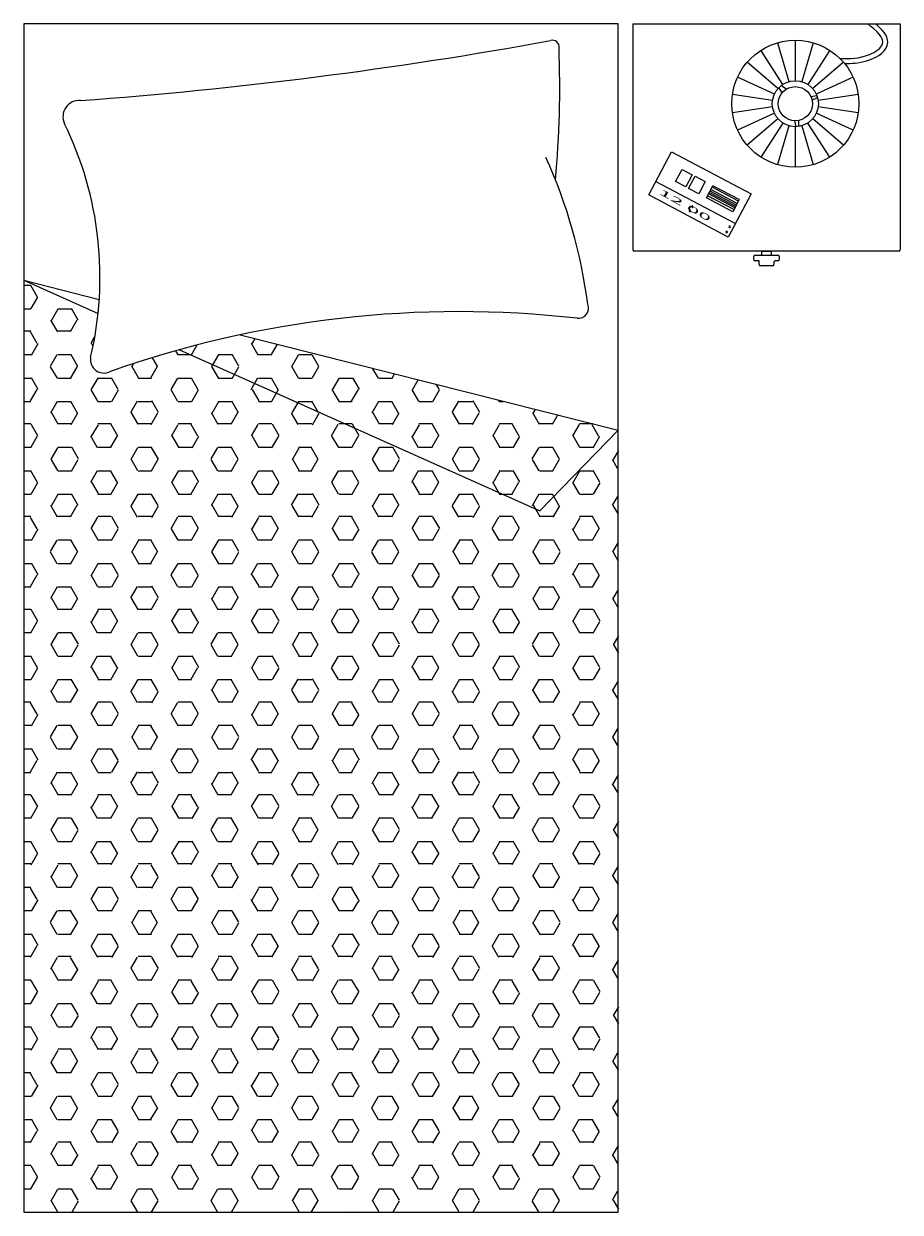
# Model space of a CAD drawing. Units: inches. Extents: x 1994 to 3075, y 3517 to 3950.
# Tile 12 of 58: x 1994.32638 to 1994.38593, y 3553.35463 to 3553.4354. Entities that reach past the tile are written whole.
import ezdxf

# ---------------------------------------------------------------- set-up
doc = ezdxf.new("R2010")
doc.units = ezdxf.units.IN
for name, color, linetype, lineweight in [('A-FURN-REFR', 8, 'Continuous', 13), ('A-FURN-REFR-PATT', 8, 'Continuous', 13), ('A-FURN-REFR-TEXT', 7, 'Continuous', 13)]:
    doc.layers.add(name, color=color, linetype=linetype, lineweight=lineweight)
doc.styles.get("Standard").update_dxf_attribs({"font": 'arial.ttf'})

msp = doc.modelspace()

# ---------------------------------------------------------------- hatches: boundary and pattern name
at = {"layer": 'A-FURN-REFR-PATT'}
h = msp.add_hatch(dxfattribs=at)
h.set_pattern_fill('HEX', color=256, scale=0.000286327845383, style=0)
h.set_pattern_definition([(180, (1995.655047321189, 3553.090100364233), (0, 0.0015745912670007), [0.0009090909090909, -0.0018181818181818]), (60, (1995.655047321189, 3553.090100364233), (0.0013636360377997, -0.0007872956335004), [0.0009090909090909, -0.0018181818181818]), (120, (1995.65413823028, 3553.090100364233), (0.0013636360377997, 0.0007872956335004), [0.0009090909090909, -0.0018181818181818])])
h.paths.add_polyline_path([(1994.326376891248, 3553.417965362907), (1994.331426744007, 3553.415710482533, -0.0305209839665435), (1994.33094919599, 3553.412850547023, 0.6531656006292759), (1994.332203126072, 3553.411747859217, -0.0174826565832849), (1994.336948128047, 3553.413245052134), (1994.361441213475, 3553.402308302044), (1994.366761804984, 3553.40777293816), (1994.366761804984, 3553.354629115022), (1994.326376891248, 3553.354629115022)])
h.paths.add_polyline_path([(1994.336948128047, 3553.413245052134, -0.0149090101017863), (1994.341069117673, 3553.414257309618), (1994.366761804984, 3553.40777293816), (1994.361441213475, 3553.402308302044)], flags=17)

# ---------------------------------------------------------------- linework, layer by layer
at = {"layer": 'A-FURN-REFR'}
for p, q in [((1994.326376891248, 3553.435398942494), (1994.326376891248, 3553.354629115022)), ((1994.366761804984, 3553.435398942494), (1994.326376891248, 3553.435398942494)), ((1994.366761804984, 3553.435398942494), (1994.326376891248, 3553.435398942494)), ((1994.326376891248, 3553.435398942494), (1994.326376891248, 3553.354629115022)), ((1994.366761804984, 3553.419954310977), (1994.366761804984, 3553.435398942494)), ((1994.367755092342, 3553.435398942494), (1994.385928303524, 3553.435398942494)), ((1994.367755092342, 3553.435398942494), (1994.385928303524, 3553.435398942494)), ((1994.367755092342, 3553.435398942494), (1994.367755092342, 3553.420048816135)), ((1994.385928303524, 3553.435398942494), (1994.385928303524, 3553.420048816135)), ((1994.37758513782, 3553.434108248894), (1994.3783607243, 3553.431466843914)), ((1994.378801208797, 3553.434283093505), (1994.378801208797, 3553.431530176024)), ((1994.378801208797, 3553.434283093505), (1994.378801208797, 3553.431530176024)), ((1994.380017279775, 3553.434108248894), (1994.379241693294, 3553.431466843914)), ((1994.377955925238, 3553.431281978377), (1994.376467585681, 3553.433597879934)), ((1994.381134831914, 3553.433597879934), (1994.379646492356, 3553.431281978377)), ((1994.377619606023, 3553.430990556118), (1994.375539089808, 3553.43279333368)), ((1994.382063327786, 3553.43279333368), (1994.379982811572, 3553.430990556118)), ((1994.377379013236, 3553.430616186435), (1994.374874871415, 3553.431759789686)), ((1994.382727546179, 3553.431759789686), (1994.380223404358, 3553.430616186435)), ((1994.377906583764, 3553.430702690964), (1994.377682333013, 3553.431058754159)), ((1994.37818918526, 3553.430950295253), (1994.377831559145, 3553.43119317567)), ((1994.377253638276, 3553.430189198535), (1994.374528741526, 3553.430580979541)), ((1994.379853427406, 3553.430451341029), (1994.380263656544, 3553.430519620496)), ((1994.379932556524, 3553.430215893215), (1994.380308524229, 3553.430382003528)), ((1994.383073676068, 3553.430580979541), (1994.380348779318, 3553.430189198535)), ((1994.377253638276, 3553.429744184436), (1994.374528741526, 3553.42935240343)), ((1994.377379013236, 3553.429317196535), (1994.374874871415, 3553.428173593284)), ((1994.382727546179, 3553.428173593284), (1994.380223404358, 3553.429317196535)), ((1994.383073676068, 3553.42935240343), (1994.380348779318, 3553.429744184436)), ((1994.377619606023, 3553.428942826852), (1994.375539089808, 3553.42714004929)), ((1994.377955925238, 3553.428651404593), (1994.376467585681, 3553.426335503037)), ((1994.3783607243, 3553.428466539056), (1994.37758513782, 3553.425825134076)), ((1994.378743486907, 3553.428809661941), (1994.378845482151, 3553.428403833919)), ((1994.378801208797, 3553.428403206946), (1994.378801208797, 3553.425650289465)), ((1994.378801208797, 3553.428403206946), (1994.378801208797, 3553.425650289465)), ((1994.379011771668, 3553.428827519655), (1994.379008923688, 3553.428417066231)), ((1994.379241693294, 3553.428466539056), (1994.380017279775, 3553.425825134076)), ((1994.381134831914, 3553.426335503037), (1994.379646492356, 3553.428651404593)), ((1994.382063327786, 3553.42714004929), (1994.379982811572, 3553.428942826852)), ((1994.368838165847, 3553.423772216742), (1994.370392794544, 3553.426704832027)), ((1994.370392794544, 3553.426704832027), (1994.375801800186, 3553.423837427142)), ((1994.370669037243, 3553.42468001607), (1994.37110664931, 3553.425505517258)), ((1994.37110664931, 3553.425505517258), (1994.371790582883, 3553.425142952566)), ((1994.371790582883, 3553.425142952566), (1994.371352970816, 3553.424317451378)), ((1994.371549513063, 3553.424213261025), (1994.37198712513, 3553.425038762214)), ((1994.37198712513, 3553.425038762214), (1994.372671058703, 3553.424676197522)), ((1994.369322787749, 3553.424686396186), (1994.374731793391, 3553.421818991302)), ((1994.371352970816, 3553.424317451378), (1994.370669037243, 3553.42468001607)), ((1994.372233446636, 3553.423850696333), (1994.371549513063, 3553.424213261025)), ((1994.372671058703, 3553.424676197522), (1994.372233446636, 3553.423850696333)), ((1994.372764783426, 3553.423569025762), (1994.373202395493, 3553.42439452695)), ((1994.374853280689, 3553.423193238081), (1994.373067436778, 3553.42413994398)), ((1994.374936407988, 3553.423350047476), (1994.373150564076, 3553.424296753377)), ((1994.374988239404, 3553.423447821051), (1994.373202395493, 3553.42439452695)), ((1994.374247171489, 3553.420904811857), (1994.368838165847, 3553.423772216742)), ((1994.374550627337, 3553.422622319863), (1994.372764783426, 3553.423569025762)), ((1994.374626875732, 3553.422766153055), (1994.372841031821, 3553.423712858954)), ((1994.374697331562, 3553.422899059289), (1994.372911487651, 3553.423845765188)), ((1994.374742012032, 3553.422983343484), (1994.372956168122, 3553.423930049385)), ((1994.374793995369, 3553.423081403636), (1994.373008151457, 3553.424028109537)), ((1994.375801800186, 3553.423837427142), (1994.374247171489, 3553.420904811857)), ((1994.374988239404, 3553.423447821051), (1994.374550627337, 3553.422622319863)), ((1994.366761804984, 3553.354629115022), (1994.366761804984, 3553.419954310977)), ((1994.366761804984, 3553.354629115022), (1994.366761804984, 3553.419954310977)), ((1994.385833798365, 3553.419954310977), (1994.367849597501, 3553.419954310977)), ((1994.375979972456, 3553.419378677088), (1994.375979972456, 3553.419589286335)), ((1994.376074477615, 3553.419683791493), (1994.377608918251, 3553.419683791493)), ((1994.376522792531, 3553.419683791493), (1994.376522792531, 3553.419954310977)), ((1994.376522792531, 3553.419954310977), (1994.377160603335, 3553.419954310977)), ((1994.377160603335, 3553.419954310977), (1994.377160603335, 3553.419683791493)), ((1994.37770342341, 3553.419589286335), (1994.37770342341, 3553.419378677088)), ((1994.376336541438, 3553.41928417193), (1994.376074477615, 3553.41928417193)), ((1994.376336541438, 3553.419032410963), (1994.376336541438, 3553.41928417193)), ((1994.37725234927, 3553.418937905804), (1994.376431046596, 3553.418937905804)), ((1994.377346854428, 3553.419189666771), (1994.377346854428, 3553.419032410963)), ((1994.377608918251, 3553.41928417193), (1994.377441359587, 3553.41928417193)), ((1994.326376891248, 3553.417965362907), (1994.331507730061, 3553.416670431616)), ((1994.326376891248, 3553.417965362907), (1994.331426744007, 3553.415710482533)), ((1994.341069117673, 3553.414257309618), (1994.366772660239, 3553.407770198488)), ((1994.336948128047, 3553.413245052134), (1994.361441213475, 3553.402308302044)), ((1994.361441213475, 3553.402308302044), (1994.366761804984, 3553.40777293816)), ((1994.326376891248, 3553.354629115022), (1994.366761804984, 3553.354629115022)), ((1994.326376891248, 3553.354629115022), (1994.366761804984, 3553.354629115022))]:
    msp.add_line(p, q, dxfattribs=at)
for radius in [0.0043164020201009, 0.0015634845390022, 0.0011584684638608]:
    msp.add_circle((1994.378801208797, 3553.429966691485), radius, dxfattribs=at)
for centre, radius, start, end in [((1994.308346638976, 3553.728998438725), 0.2996159645214513, 274.1894661396486, 280.345956739574), ((1994.362305122703, 3553.433831407612), 0.0004482907065646, 350.157018905503, 109.5558986651033), ((1994.293858092433, 3553.43120871463), 0.0689357559366832, 354.6669486061241, 2.116631318036676), ((1994.330138900409, 3553.429088750875), 0.0010985341214448, 84.97952421387143, 205.9936625746376), ((1994.307783814709, 3553.418188507773), 0.0237724360313189, 346.680428679662, 25.99366257463764), ((1994.329755793335, 3553.411758672162), 0.0352435291682938, 7.457332088483644, 24.3977020455474), ((1994.371636141821, 3553.422690145915), 5.53897148363e-05, 90, 270), ((1994.371636141821, 3553.422690145915), 5.53897148363e-05, 270, 90), ((1994.37180825677, 3553.422970060961), 5.53897148363e-05, 90, 270), ((1994.37180825677, 3553.422970060961), 5.53897148363e-05, 270, 90), ((1994.374133474014, 3553.421252658023), 5.53897148363e-05, 90, 270), ((1994.374133474014, 3553.421252658023), 5.53897148363e-05, 270, 90), ((1994.374333601732, 3553.421602254547), 5.53897148363e-05, 90, 270), ((1994.374333601732, 3553.421602254547), 5.53897148363e-05, 270, 90), ((1994.367849597501, 3553.420048816135), 9.45051583805e-05, 180, 270), ((1994.376074477615, 3553.419589286335), 9.45051583805e-05, 90, 180), ((1994.376074477615, 3553.419378677088), 9.45051583805e-05, 180, 270), ((1994.377608918251, 3553.419589286335), 9.45051583805e-05, 0, 90), ((1994.377608918251, 3553.419378677088), 9.45051583805e-05, 270, 0), ((1994.385833798365, 3553.420048816135), 9.45051583805e-05, 270, 0), ((1994.376431046596, 3553.419032410963), 9.45051583805e-05, 180, 270), ((1994.37725234927, 3553.419032410963), 9.45051583805e-05, 270, 0), ((1994.377441359587, 3553.419189666771), 9.45051583805e-05, 90, 180), ((1994.364066261875, 3553.416067965212), 0.0006880002040652, 263.537978316425, 22.64447096621987), ((1994.35597877168, 3553.344664206115), 0.0711723108928985, 83.53797831642504, 109.5152363664946), ((1994.331818156815, 3553.412574390524), 0.0009117868872928, 171.3346578780885, 294.9744503598286)]:
    msp.add_arc(centre, radius, start, end, dxfattribs=at)
for points, knots in [([(1994.381838208368, 3553.433033931288), (1994.382491457716, 3553.433021698712), (1994.383513929715, 3553.433014861758), (1994.385241084575, 3553.434139388716), (1994.384297393522, 3553.434931305883), (1994.383731944177, 3553.435398942494)], [0, 0, 0, 0, 0.0020194675197693, 0.0031659294013046, 0.0048546887779192, 0.0048546887779192, 0.0048546887779192, 0.0048546887779192]), ([(1994.382138850867, 3553.432703746802), (1994.382611100438, 3553.432699897468), (1994.383112337832, 3553.43272016468), (1994.384178987074, 3553.433053333693), (1994.384851069915, 3553.433305061542), (1994.385212843929, 3553.434459620106), (1994.384812874639, 3553.434879894214), (1994.384367255243, 3553.435287773298), (1994.384303663627, 3553.43534363005), (1994.384239148789, 3553.435398942494)], [0.0077183477163671, 0.0077183477163671, 0.0077183477163671, 0.0077183477163671, 0.0428867239757183, 0.0428867239757183, 0.0785443346356031, 0.0785443346356031, 0.1084777623087474, 0.1084777623087474, 0.1132872864949097, 0.1132872864949097, 0.1132872864949097, 0.1132872864949097])]:
    msp.add_open_spline(points, degree=3, knots=knots, dxfattribs=at)

# ---------------------------------------------------------------- texts
at = {"layer": 'A-FURN-REFR-TEXT', "width": 3}
msp.add_text('12 00', height=0.000395772154613, rotation=330.6435157060532, dxfattribs=at).set_placement((1994.369485239311, 3553.423870823898))

doc.saveas('drawing.dxf')
